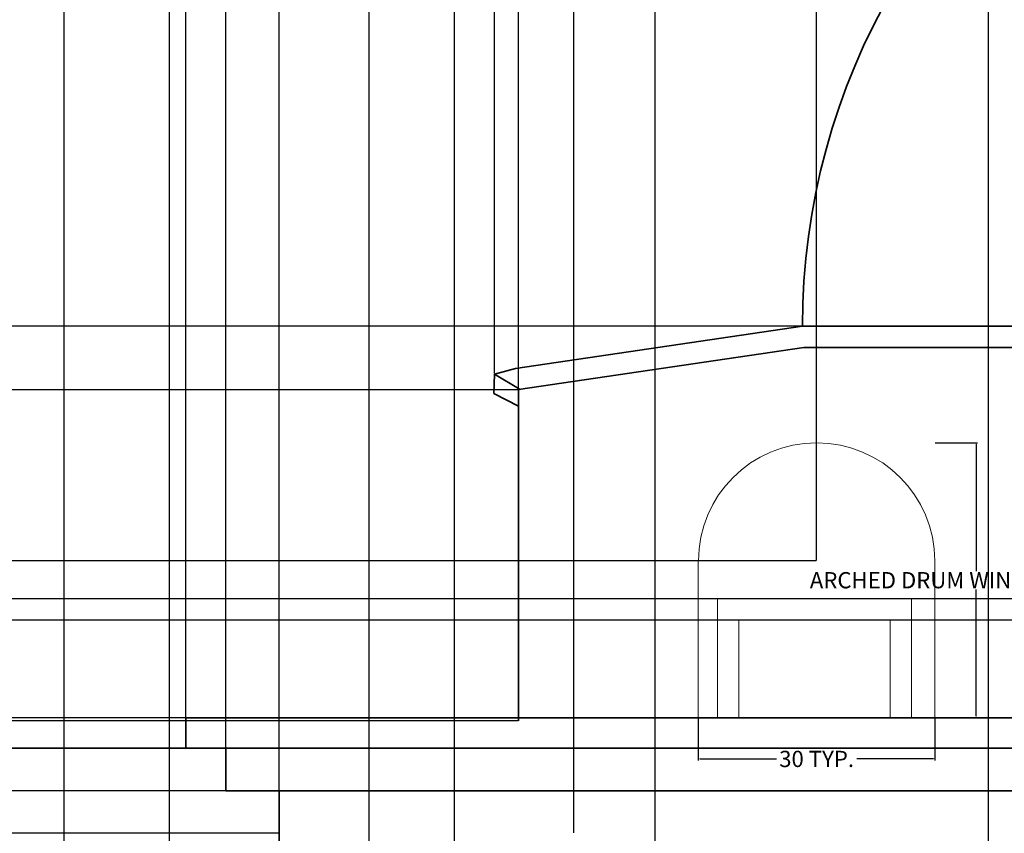
# Model space of a CAD drawing. Units: inches. Extents: x 14 to 859, y 52 to 711.
# Tile 6 of 11: x 244 to 368, y 504 to 608. Entities that reach past the tile are written whole.
import ezdxf

# ---------------------------------------------------------------- set-up
doc = ezdxf.new("R2010")
doc.units = ezdxf.units.IN
doc.header["$MEASUREMENT"] = 0
for name, color, linetype, lineweight in [('A-ANNO-DIMS', 2, 'Continuous', 18), ('A-ELEV', 7, 'Continuous', 35), ('A-GLAZ', 4, 'Continuous', 18), ('A-ROOF', 7, 'Continuous', 35)]:
    doc.layers.add(name, color=color, linetype=linetype, lineweight=lineweight)
doc.styles.get("Standard").update_dxf_attribs({"font": 'arial.ttf'})
doc.dimstyles.get("Standard").update_dxf_attribs({"dimtxt": 2.0625, "dimasz": 0.18, "dimexe": 0.18, "dimexo": 0.0625, "dimgap": 0.09, "dimtad": 0, "dimtih": 1, "dimtoh": 1, "dimdec": 4, "dimzin": 0, "dimdsep": 46, "dimlunit": 4, "dimtxsty": 'Standard', "dimcen": 0.09, "dimadec": 0, "dimazin": 0, "dimtfac": 1, "dimtdec": 4, "dimtofl": 0, "dimtmove": 0, "dimatfit": 3, "dimfxl": 1, "dimtolj": 1, "dimtzin": 0, "dimarcsym": 0})

# ---------------------------------------------------------------- blocks, each defined once
blk = doc.blocks.new('WIN-DRUM-ARCHED')
for p, q in [((329.67, 519.05), (329.67, 538.94)), ((359.68, 519.05), (359.68, 538.94))]:
    blk.add_line(p, q)
for points in [[(332.09, 519.05), (332.09, 534.15), (356.71, 534.15), (356.71, 519.05)], [(334.8, 519.05), (334.8, 531.45), (354.01, 531.45), (354.01, 519.05)]]:
    blk.add_lwpolyline(points)
blk.add_arc((344.68, 538.94), 15, 0, 180)
blk = doc.blocks.new('*D11')
at = {"layer": 'A-ANNO-DIMS', "color": 0, "lineweight": -2, "transparency": 16777216}
for p, q in [((359.74, 553.94), (365.09, 553.94)), ((364.91, 553.76), (364.91, 537.66)), ((364.91, 519.23), (364.91, 535.34)), ((359.74, 519.05), (365.09, 519.05))]:
    blk.add_line(p, q, dxfattribs=at)
at = {"layer": 'A-ANNO-DIMS', "color": 0, "transparency": 16777216}
for points in [[(364.88, 553.76), (364.94, 553.76), (364.91, 553.94)], [(364.88, 519.23), (364.94, 519.23), (364.91, 519.05)]]:
    blk.add_solid(points, dxfattribs=at)
at = {"layer": 'Defpoints', "color": 0, "transparency": 16777216}
for p in [(359.68, 553.94), (364.91, 553.94), (359.68, 519.05)]:
    blk.add_point(p, dxfattribs=at)
at = {"layer": 'A-ANNO-DIMS', "color": 0, "transparency": 16777216, "insert": (364.91, 536.5), "char_height": 2.0625, "attachment_point": 5}
blk.add_mtext('\\A1;ARCHED DRUM WINDOW 35 TYP.', dxfattribs=at)
blk = doc.blocks.new('*D12')
at = {"layer": 'A-ANNO-DIMS', "color": 0, "lineweight": -2, "transparency": 16777216}
for p, q in [((329.67, 518.99), (329.67, 513.64)), ((359.68, 518.99), (359.68, 513.64)), ((329.85, 513.82), (339.57, 513.82)), ((359.5, 513.82), (349.79, 513.82))]:
    blk.add_line(p, q, dxfattribs=at)
at = {"layer": 'A-ANNO-DIMS', "color": 0, "transparency": 16777216}
for points in [[(329.85, 513.85), (329.85, 513.79), (329.67, 513.82)], [(359.5, 513.85), (359.5, 513.79), (359.68, 513.82)]]:
    blk.add_solid(points, dxfattribs=at)
at = {"layer": 'Defpoints', "color": 0, "transparency": 16777216}
for p in [(329.67, 519.05), (359.68, 519.05), (359.68, 513.82)]:
    blk.add_point(p, dxfattribs=at)
at = {"layer": 'A-ANNO-DIMS', "color": 0, "transparency": 16777216, "insert": (344.68, 513.82), "char_height": 2.0625, "attachment_point": 5}
blk.add_mtext('\\A1;30 TYP.', dxfattribs=at)
blk = doc.blocks.new('*D13')
at = {"layer": 'A-ANNO-DIMS', "color": 0, "lineweight": -2, "transparency": 16777216}
for p, q in [((60.78, 339.73), (60.78, 709.71)), ((811.55, 339.73), (811.55, 709.71)), ((60.96, 709.53), (432.6, 709.53)), ((811.37, 709.53), (439.73, 709.53))]:
    blk.add_line(p, q, dxfattribs=at)
at = {"layer": 'A-ANNO-DIMS', "color": 0, "transparency": 16777216}
for points in [[(60.96, 709.56), (60.96, 709.5), (60.78, 709.53)], [(811.37, 709.56), (811.37, 709.5), (811.55, 709.53)]]:
    blk.add_solid(points, dxfattribs=at)
at = {"layer": 'Defpoints', "color": 0, "transparency": 16777216}
for p in [(811.55, 709.53), (60.78, 339.66), (811.55, 339.66)]:
    blk.add_point(p, dxfattribs=at)
at = {"layer": 'A-ANNO-DIMS', "color": 0, "transparency": 16777216, "insert": (436.17, 709.53), "char_height": 2.062, "attachment_point": 5}
blk.add_mtext('\\A1;750.8', dxfattribs=at)
blk = doc.blocks.new('*D16')
at = {"layer": 'A-ANNO-DIMS', "color": 0, "lineweight": -2, "transparency": 16777216}
for p, q in [((429.96, 670.76), (17.7, 670.76)), ((17.88, 670.58), (17.88, 384.41)), ((17.88, 95.97), (17.88, 382.14)), ((60.72, 95.79), (17.7, 95.79))]:
    blk.add_line(p, q, dxfattribs=at)
at = {"layer": 'A-ANNO-DIMS', "color": 0, "transparency": 16777216}
for points in [[(17.85, 670.58), (17.91, 670.58), (17.88, 670.76)], [(17.85, 95.97), (17.91, 95.97), (17.88, 95.79)]]:
    blk.add_solid(points, dxfattribs=at)
at = {"layer": 'Defpoints', "color": 0, "transparency": 16777216}
for p in [(17.88, 670.76), (430.02, 670.76), (60.78, 95.79)]:
    blk.add_point(p, dxfattribs=at)
at = {"layer": 'A-ANNO-DIMS', "color": 0, "transparency": 16777216, "insert": (17.88, 383.28), "char_height": 2.062, "attachment_point": 5}
blk.add_mtext('\\A1;575', dxfattribs=at)
blk = doc.blocks.new('*D21')
at = {"layer": 'A-ANNO-DIMS', "color": 0, "lineweight": -2, "transparency": 16777216}
for p, q in [((287.89, 352.49), (287.89, 709.71)), ((298.73, 341.73), (298.73, 709.71)), ((288.07, 709.53), (289.04, 709.53)), ((298.55, 709.53), (297.59, 709.53))]:
    blk.add_line(p, q, dxfattribs=at)
at = {"layer": 'A-ANNO-DIMS', "color": 0, "transparency": 16777216}
for points in [[(288.07, 709.56), (288.07, 709.5), (287.89, 709.53)], [(298.55, 709.56), (298.55, 709.5), (298.73, 709.53)]]:
    blk.add_solid(points, dxfattribs=at)
at = {"layer": 'Defpoints', "color": 0, "transparency": 16777216}
for p in [(298.73, 709.53), (287.89, 352.43), (298.73, 341.67)]:
    blk.add_point(p, dxfattribs=at)
at = {"layer": 'A-ANNO-DIMS', "color": 0, "transparency": 16777216, "insert": (293.31, 709.53), "char_height": 2.062, "attachment_point": 5}
blk.add_mtext('\\A1;10.837', dxfattribs=at)
blk = doc.blocks.new('*D22')
at = {"layer": 'A-ANNO-DIMS', "color": 0, "lineweight": -2, "transparency": 16777216}
for p, q in [((298.73, 341.73), (298.73, 709.71)), ((576.51, 341.73), (576.51, 709.71)), ((298.91, 709.53), (434.03, 709.53)), ((576.33, 709.53), (441.21, 709.53))]:
    blk.add_line(p, q, dxfattribs=at)
at = {"layer": 'A-ANNO-DIMS', "color": 0, "transparency": 16777216}
for points in [[(298.91, 709.56), (298.91, 709.5), (298.73, 709.53)], [(576.33, 709.56), (576.33, 709.5), (576.51, 709.53)]]:
    blk.add_solid(points, dxfattribs=at)
at = {"layer": 'Defpoints', "color": 0, "transparency": 16777216}
for p in [(576.51, 709.53), (298.73, 341.67), (576.51, 341.67)]:
    blk.add_point(p, dxfattribs=at)
at = {"layer": 'A-ANNO-DIMS', "color": 0, "transparency": 16777216, "insert": (437.62, 709.53), "char_height": 2.062, "attachment_point": 5}
blk.add_mtext('\\A1;277.8', dxfattribs=at)
blk = doc.blocks.new('*D66')
at = {"layer": 'A-ANNO-DIMS', "color": 0, "lineweight": -2, "transparency": 16777216}
for p, q in [((223.53, 404.43), (223.53, 709.71)), ((249.19, 404.43), (249.19, 709.71)), ((223.71, 709.53), (232.77, 709.53)), ((249.01, 709.53), (239.95, 709.53))]:
    blk.add_line(p, q, dxfattribs=at)
at = {"layer": 'A-ANNO-DIMS', "color": 0, "transparency": 16777216}
for points in [[(223.71, 709.56), (223.71, 709.5), (223.53, 709.53)], [(249.01, 709.56), (249.01, 709.5), (249.19, 709.53)]]:
    blk.add_solid(points, dxfattribs=at)
at = {"layer": 'Defpoints', "color": 0, "transparency": 16777216}
for p in [(249.19, 709.53), (223.53, 404.37), (249.19, 404.37)]:
    blk.add_point(p, dxfattribs=at)
at = {"layer": 'A-ANNO-DIMS', "color": 0, "transparency": 16777216, "insert": (236.36, 709.53), "char_height": 2.062, "attachment_point": 5}
blk.add_mtext('\\A1;25.67', dxfattribs=at)
blk = doc.blocks.new('*D67')
at = {"layer": 'A-ANNO-DIMS', "color": 0, "lineweight": -2, "transparency": 16777216}
for p, q in [((249.19, 404.43), (249.19, 709.71)), ((262.58, 404.43), (262.58, 709.71)), ((249.37, 709.53), (252.41, 709.53)), ((262.4, 709.53), (259.36, 709.53))]:
    blk.add_line(p, q, dxfattribs=at)
at = {"layer": 'A-ANNO-DIMS', "color": 0, "transparency": 16777216}
for points in [[(249.37, 709.56), (249.37, 709.5), (249.19, 709.53)], [(262.4, 709.56), (262.4, 709.5), (262.58, 709.53)]]:
    blk.add_solid(points, dxfattribs=at)
at = {"layer": 'Defpoints', "color": 0, "transparency": 16777216}
for p in [(262.58, 709.53), (249.19, 404.37), (262.58, 404.37)]:
    blk.add_point(p, dxfattribs=at)
at = {"layer": 'A-ANNO-DIMS', "color": 0, "transparency": 16777216, "insert": (255.89, 709.53), "char_height": 2.062, "attachment_point": 5}
blk.add_mtext('\\A1;13.39', dxfattribs=at)
blk = doc.blocks.new('*D87')
at = {"layer": 'A-ANNO-DIMS', "color": 0, "lineweight": -2, "transparency": 16777216}
for p, q in [((276.44, 504.38), (17.7, 504.38)), ((17.88, 504.2), (17.88, 476.81)), ((17.88, 447.13), (17.88, 474.52)), ((366.44, 446.95), (17.7, 446.95))]:
    blk.add_line(p, q, dxfattribs=at)
at = {"layer": 'A-ANNO-DIMS', "color": 0, "transparency": 16777216}
for points in [[(17.85, 504.2), (17.91, 504.2), (17.88, 504.38)], [(17.85, 447.13), (17.91, 447.13), (17.88, 446.95)]]:
    blk.add_solid(points, dxfattribs=at)
at = {"layer": 'Defpoints', "color": 0, "transparency": 16777216}
for p in [(17.88, 504.38), (276.5, 504.38), (366.51, 446.95)]:
    blk.add_point(p, dxfattribs=at)
at = {"layer": 'A-ANNO-DIMS', "color": 0, "transparency": 16777216, "insert": (17.88, 475.67), "char_height": 2.062, "attachment_point": 5}
blk.add_mtext('\\A1;57.43', dxfattribs=at)
blk = doc.blocks.new('*D88')
at = {"layer": 'A-ANNO-DIMS', "color": 0, "lineweight": -2, "transparency": 16777216}
for p, q in [((276.44, 509.79), (17.7, 509.79)), ((17.88, 509.61), (17.88, 508.23)), ((17.88, 504.56), (17.88, 505.94)), ((276.44, 504.38), (17.7, 504.38))]:
    blk.add_line(p, q, dxfattribs=at)
at = {"layer": 'A-ANNO-DIMS', "color": 0, "transparency": 16777216}
for points in [[(17.85, 509.61), (17.91, 509.61), (17.88, 509.79)], [(17.85, 504.56), (17.91, 504.56), (17.88, 504.38)]]:
    blk.add_solid(points, dxfattribs=at)
at = {"layer": 'Defpoints', "color": 0, "transparency": 16777216}
for p in [(17.88, 509.79), (276.5, 509.79), (276.5, 504.38)]:
    blk.add_point(p, dxfattribs=at)
at = {"layer": 'A-ANNO-DIMS', "color": 0, "transparency": 16777216, "insert": (17.88, 507.09), "char_height": 2.062, "attachment_point": 5}
blk.add_mtext('\\A1;5.409', dxfattribs=at)
blk = doc.blocks.new('*D89')
at = {"layer": 'A-ANNO-DIMS', "color": 0, "lineweight": -2, "transparency": 16777216}
for p, q in [((269.65, 515.2), (17.7, 515.2)), ((17.88, 515.02), (17.88, 513.64)), ((17.88, 509.97), (17.88, 511.35)), ((269.65, 509.79), (17.7, 509.79))]:
    blk.add_line(p, q, dxfattribs=at)
at = {"layer": 'A-ANNO-DIMS', "color": 0, "transparency": 16777216}
for points in [[(17.85, 515.02), (17.91, 515.02), (17.88, 515.2)], [(17.85, 509.97), (17.91, 509.97), (17.88, 509.79)]]:
    blk.add_solid(points, dxfattribs=at)
at = {"layer": 'Defpoints', "color": 0, "transparency": 16777216}
for p in [(17.88, 515.2), (269.71, 515.2), (269.71, 509.79)]:
    blk.add_point(p, dxfattribs=at)
at = {"layer": 'A-ANNO-DIMS', "color": 0, "transparency": 16777216, "insert": (17.88, 512.49), "char_height": 2.062, "attachment_point": 5}
blk.add_mtext('\\A1;5.409', dxfattribs=at)
blk = doc.blocks.new('*D90')
at = {"layer": 'A-ANNO-DIMS', "color": 0, "lineweight": -2, "transparency": 16777216}
for p, q in [((264.56, 519.05), (17.7, 519.05)), ((17.88, 518.87), (17.88, 518.24)), ((264.56, 515.14), (17.7, 515.14)), ((17.88, 515.32), (17.88, 515.95))]:
    blk.add_line(p, q, dxfattribs=at)
at = {"layer": 'A-ANNO-DIMS', "color": 0, "transparency": 16777216}
for points in [[(17.85, 518.87), (17.91, 518.87), (17.88, 519.05)], [(17.85, 515.32), (17.91, 515.32), (17.88, 515.14)]]:
    blk.add_solid(points, dxfattribs=at)
at = {"layer": 'Defpoints', "color": 0, "transparency": 16777216}
for p in [(17.88, 519.05), (264.63, 519.05), (264.63, 515.14)]:
    blk.add_point(p, dxfattribs=at)
at = {"layer": 'A-ANNO-DIMS', "color": 0, "transparency": 16777216, "insert": (17.88, 517.1), "char_height": 2.062, "attachment_point": 5}
blk.add_mtext('\\A1;3.91', dxfattribs=at)
blk = doc.blocks.new('*D91')
at = {"layer": 'A-ANNO-DIMS', "color": 0, "lineweight": -2, "transparency": 16777216}
for p, q in [((306.8, 560.68), (17.7, 560.68)), ((17.88, 560.5), (17.88, 541.01)), ((17.88, 519.23), (17.88, 538.72)), ((264.56, 519.05), (17.7, 519.05))]:
    blk.add_line(p, q, dxfattribs=at)
at = {"layer": 'A-ANNO-DIMS', "color": 0, "transparency": 16777216}
for points in [[(17.85, 560.5), (17.91, 560.5), (17.88, 560.68)], [(17.85, 519.23), (17.91, 519.23), (17.88, 519.05)]]:
    blk.add_solid(points, dxfattribs=at)
at = {"layer": 'Defpoints', "color": 0, "transparency": 16777216}
for p in [(17.88, 560.68), (306.86, 560.68), (264.63, 519.05)]:
    blk.add_point(p, dxfattribs=at)
at = {"layer": 'A-ANNO-DIMS', "color": 0, "transparency": 16777216, "insert": (17.88, 539.87), "char_height": 2.062, "attachment_point": 5}
blk.add_mtext('\\A1;41.63', dxfattribs=at)
blk = doc.blocks.new('*D92')
at = {"layer": 'A-ANNO-DIMS', "color": 0, "lineweight": -2, "transparency": 16777216}
for p, q in [((342.81, 568.74), (17.7, 568.74)), ((17.88, 568.56), (17.88, 565.85)), ((17.88, 560.86), (17.88, 563.57)), ((306.8, 560.68), (17.7, 560.68))]:
    blk.add_line(p, q, dxfattribs=at)
at = {"layer": 'A-ANNO-DIMS', "color": 0, "transparency": 16777216}
for points in [[(17.85, 568.56), (17.91, 568.56), (17.88, 568.74)], [(17.85, 560.86), (17.91, 560.86), (17.88, 560.68)]]:
    blk.add_solid(points, dxfattribs=at)
at = {"layer": 'Defpoints', "color": 0, "transparency": 16777216}
for p in [(17.88, 568.74), (342.87, 568.74), (306.86, 560.68)]:
    blk.add_point(p, dxfattribs=at)
at = {"layer": 'A-ANNO-DIMS', "color": 0, "transparency": 16777216, "insert": (17.88, 564.71), "char_height": 2.062, "attachment_point": 5}
blk.add_mtext('\\A1;8.055', dxfattribs=at)
blk = doc.blocks.new('*D93')
at = {"layer": 'A-ANNO-DIMS', "color": 0, "lineweight": -2, "transparency": 16777216}
for p, q in [((429.22, 654.01), (17.7, 654.01)), ((17.88, 653.83), (17.88, 612.51)), ((17.88, 568.92), (17.88, 610.23)), ((342.81, 568.74), (17.7, 568.74))]:
    blk.add_line(p, q, dxfattribs=at)
at = {"layer": 'A-ANNO-DIMS', "color": 0, "transparency": 16777216}
for points in [[(17.85, 653.83), (17.91, 653.83), (17.88, 654.01)], [(17.85, 568.92), (17.91, 568.92), (17.88, 568.74)]]:
    blk.add_solid(points, dxfattribs=at)
at = {"layer": 'Defpoints', "color": 0, "transparency": 16777216}
for p in [(17.88, 654.01), (429.29, 654.01), (342.87, 568.74)]:
    blk.add_point(p, dxfattribs=at)
at = {"layer": 'A-ANNO-DIMS', "color": 0, "transparency": 16777216, "insert": (17.88, 611.37), "char_height": 2.062, "attachment_point": 5}
blk.add_mtext('\\A1;85.27', dxfattribs=at)
blk = doc.blocks.new('*D95')
at = {"layer": 'A-ANNO-DIMS', "color": 0, "lineweight": -2, "transparency": 16777216}
for p, q in [((276.5, 504.44), (276.5, 709.71)), ((313.86, 504.44), (313.86, 709.71)), ((276.68, 709.53), (290.81, 709.53)), ((313.68, 709.53), (299.55, 709.53))]:
    blk.add_line(p, q, dxfattribs=at)
at = {"layer": 'A-ANNO-DIMS', "color": 0, "transparency": 16777216}
for points in [[(276.68, 709.56), (276.68, 709.5), (276.5, 709.53)], [(313.68, 709.56), (313.68, 709.5), (313.86, 709.53)]]:
    blk.add_solid(points, dxfattribs=at)
at = {"layer": 'Defpoints', "color": 0, "transparency": 16777216}
for p in [(313.86, 709.53), (276.5, 504.38), (313.86, 504.38)]:
    blk.add_point(p, dxfattribs=at)
at = {"layer": 'A-ANNO-DIMS', "color": 0, "transparency": 16777216, "insert": (295.18, 709.53), "char_height": 2.062, "attachment_point": 5}
blk.add_mtext('\\A1;37.356', dxfattribs=at)
blk = doc.blocks.new('*D96')
at = {"layer": 'A-ANNO-DIMS', "color": 0, "lineweight": -2, "transparency": 16777216}
for p, q in [((313.86, 504.44), (313.86, 709.71)), ((366.51, 447.01), (366.51, 709.71)), ((314.04, 709.53), (336.61, 709.53)), ((366.33, 709.53), (343.76, 709.53))]:
    blk.add_line(p, q, dxfattribs=at)
at = {"layer": 'A-ANNO-DIMS', "color": 0, "transparency": 16777216}
for points in [[(314.04, 709.56), (314.04, 709.5), (313.86, 709.53)], [(366.33, 709.56), (366.33, 709.5), (366.51, 709.53)]]:
    blk.add_solid(points, dxfattribs=at)
at = {"layer": 'Defpoints', "color": 0, "transparency": 16777216}
for p in [(366.51, 709.53), (313.86, 504.38), (366.51, 446.95)]:
    blk.add_point(p, dxfattribs=at)
at = {"layer": 'A-ANNO-DIMS', "color": 0, "transparency": 16777216, "insert": (340.18, 709.53), "char_height": 2.062, "attachment_point": 5}
blk.add_mtext('\\A1;52.65', dxfattribs=at)
blk = doc.blocks.new('*D97')
at = {"layer": 'A-ANNO-DIMS', "color": 0, "lineweight": -2, "transparency": 16777216}
for p, q in [((366.51, 447.01), (366.51, 709.71)), ((433.06, 447.01), (433.06, 709.71)), ((366.69, 709.53), (396.2, 709.53)), ((432.88, 709.53), (403.37, 709.53))]:
    blk.add_line(p, q, dxfattribs=at)
at = {"layer": 'A-ANNO-DIMS', "color": 0, "transparency": 16777216}
for points in [[(366.69, 709.56), (366.69, 709.5), (366.51, 709.53)], [(432.88, 709.56), (432.88, 709.5), (433.06, 709.53)]]:
    blk.add_solid(points, dxfattribs=at)
at = {"layer": 'Defpoints', "color": 0, "transparency": 16777216}
for p in [(433.06, 709.53), (366.51, 446.95), (433.06, 446.95)]:
    blk.add_point(p, dxfattribs=at)
at = {"layer": 'A-ANNO-DIMS', "color": 0, "transparency": 16777216, "insert": (399.78, 709.53), "char_height": 2.062, "attachment_point": 5}
blk.add_mtext('\\A1;66.55', dxfattribs=at)
blk = doc.blocks.new('*D104')
at = {"layer": 'A-ANNO-DIMS', "color": 0, "lineweight": -2, "transparency": 16777216}
for p, q in [((264.63, 519.11), (264.63, 709.71)), ((269.71, 515.26), (269.71, 709.71)), ((264.81, 709.53), (269.53, 709.53)), ((269.71, 709.53), (269.89, 709.53))]:
    blk.add_line(p, q, dxfattribs=at)
at = {"layer": 'A-ANNO-DIMS', "color": 0, "transparency": 16777216}
for points in [[(264.81, 709.56), (264.81, 709.5), (264.63, 709.53)], [(269.53, 709.56), (269.53, 709.5), (269.71, 709.53)]]:
    blk.add_solid(points, dxfattribs=at)
at = {"layer": 'Defpoints', "color": 0, "transparency": 16777216}
for p in [(269.71, 709.53), (264.63, 519.05), (269.71, 515.2)]:
    blk.add_point(p, dxfattribs=at)
at = {"layer": 'A-ANNO-DIMS', "color": 0, "transparency": 16777216, "insert": (273.46, 709.53), "char_height": 2.062, "attachment_point": 5}
blk.add_mtext('\\A1;5.084', dxfattribs=at)
blk = doc.blocks.new('*D105')
at = {"layer": 'A-ANNO-DIMS', "color": 0, "lineweight": -2, "transparency": 16777216}
for p, q in [((306.86, 560.74), (306.86, 709.71)), ((549.44, 560.74), (549.44, 709.71)), ((307.04, 709.53), (424.56, 709.53)), ((549.26, 709.53), (431.74, 709.53))]:
    blk.add_line(p, q, dxfattribs=at)
at = {"layer": 'A-ANNO-DIMS', "color": 0, "transparency": 16777216}
for points in [[(307.04, 709.56), (307.04, 709.5), (306.86, 709.53)], [(549.26, 709.56), (549.26, 709.5), (549.44, 709.53)]]:
    blk.add_solid(points, dxfattribs=at)
at = {"layer": 'Defpoints', "color": 0, "transparency": 16777216}
for p in [(549.44, 709.53), (306.86, 560.68), (549.44, 560.68)]:
    blk.add_point(p, dxfattribs=at)
at = {"layer": 'A-ANNO-DIMS', "color": 0, "transparency": 16777216, "insert": (428.15, 709.53), "char_height": 2.062, "attachment_point": 5}
blk.add_mtext('\\A1;242.6', dxfattribs=at)
blk = doc.blocks.new('*D106')
at = {"layer": 'A-ANNO-DIMS', "color": 0, "lineweight": -2, "transparency": 16777216}
for p, q in [((303.82, 562.72), (303.82, 709.71)), ((306.86, 560.74), (306.86, 709.71)), ((304, 709.53), (306.68, 709.53)), ((306.86, 709.53), (307.04, 709.53))]:
    blk.add_line(p, q, dxfattribs=at)
at = {"layer": 'A-ANNO-DIMS', "color": 0, "transparency": 16777216}
for points in [[(304, 709.56), (304, 709.5), (303.82, 709.53)], [(306.68, 709.56), (306.68, 709.5), (306.86, 709.53)]]:
    blk.add_solid(points, dxfattribs=at)
at = {"layer": 'Defpoints', "color": 0, "transparency": 16777216}
for p in [(306.86, 709.53), (303.82, 562.66), (306.86, 560.68)]:
    blk.add_point(p, dxfattribs=at)
at = {"layer": 'A-ANNO-DIMS', "color": 0, "transparency": 16777216, "insert": (309.8, 709.53), "char_height": 2.062, "attachment_point": 5}
blk.add_mtext('\\A1;3.04', dxfattribs=at)
blk = doc.blocks.new('*D108')
at = {"layer": 'A-ANNO-DIMS', "color": 0, "lineweight": -2, "transparency": 16777216}
for p, q in [((264.63, 519.11), (264.63, 709.71)), ((306.86, 560.74), (306.86, 709.71)), ((264.81, 709.53), (282.13, 709.53)), ((306.68, 709.53), (289.36, 709.53))]:
    blk.add_line(p, q, dxfattribs=at)
at = {"layer": 'A-ANNO-DIMS', "color": 0, "transparency": 16777216}
for points in [[(264.81, 709.56), (264.81, 709.5), (264.63, 709.53)], [(306.68, 709.56), (306.68, 709.5), (306.86, 709.53)]]:
    blk.add_solid(points, dxfattribs=at)
at = {"layer": 'Defpoints', "color": 0, "transparency": 16777216}
for p in [(306.86, 709.53), (306.86, 560.68), (264.63, 519.05)]:
    blk.add_point(p, dxfattribs=at)
at = {"layer": 'A-ANNO-DIMS', "color": 0, "transparency": 16777216, "insert": (285.74, 709.53), "char_height": 2.062, "attachment_point": 5}
blk.add_mtext('\\A1;42.23', dxfattribs=at)
blk = doc.blocks.new('*D109')
at = {"layer": 'A-ANNO-DIMS', "color": 0, "lineweight": -2, "transparency": 16777216}
for p, q in [((269.71, 515.26), (269.71, 709.71)), ((276.5, 509.85), (276.5, 709.71)), ((269.89, 709.53), (276.32, 709.53)), ((276.5, 709.53), (276.68, 709.53))]:
    blk.add_line(p, q, dxfattribs=at)
at = {"layer": 'A-ANNO-DIMS', "color": 0, "transparency": 16777216}
for points in [[(269.89, 709.56), (269.89, 709.5), (269.71, 709.53)], [(276.32, 709.56), (276.32, 709.5), (276.5, 709.53)]]:
    blk.add_solid(points, dxfattribs=at)
at = {"layer": 'Defpoints', "color": 0, "transparency": 16777216}
for p in [(276.5, 709.53), (269.71, 515.2), (276.5, 509.79)]:
    blk.add_point(p, dxfattribs=at)
at = {"layer": 'A-ANNO-DIMS', "color": 0, "transparency": 16777216, "insert": (280.26, 709.53), "char_height": 2.062, "attachment_point": 5}
blk.add_mtext('\\A1;6.793', dxfattribs=at)
blk = doc.blocks.new('*D110')
at = {"layer": 'A-ANNO-DIMS', "color": 0, "lineweight": -2, "transparency": 16777216}
for p, q in [((306.86, 518.73), (306.86, 709.71)), ((344.68, 539), (344.68, 709.71)), ((307.04, 709.53), (322.21, 709.53)), ((344.5, 709.53), (329.33, 709.53))]:
    blk.add_line(p, q, dxfattribs=at)
at = {"layer": 'A-ANNO-DIMS', "color": 0, "transparency": 16777216}
for points in [[(307.04, 709.56), (307.04, 709.5), (306.86, 709.53)], [(344.5, 709.56), (344.5, 709.5), (344.68, 709.53)]]:
    blk.add_solid(points, dxfattribs=at)
at = {"layer": 'Defpoints', "color": 0, "transparency": 16777216}
for p in [(344.68, 709.53), (344.68, 538.94), (306.86, 518.67)]:
    blk.add_point(p, dxfattribs=at)
at = {"layer": 'A-ANNO-DIMS', "color": 0, "transparency": 16777216, "insert": (325.77, 709.53), "char_height": 2.062, "attachment_point": 5}
blk.add_mtext('\\A1;37.82', dxfattribs=at)
blk = doc.blocks.new('*D111')
at = {"layer": 'A-ANNO-DIMS', "color": 0, "lineweight": -2, "transparency": 16777216}
for p, q in [((344.68, 539), (344.68, 709.71)), ((424.02, 539), (424.02, 709.71)), ((344.86, 709.53), (380.79, 709.53)), ((423.84, 709.53), (387.91, 709.53))]:
    blk.add_line(p, q, dxfattribs=at)
at = {"layer": 'A-ANNO-DIMS', "color": 0, "transparency": 16777216}
for points in [[(344.86, 709.56), (344.86, 709.5), (344.68, 709.53)], [(423.84, 709.56), (423.84, 709.5), (424.02, 709.53)]]:
    blk.add_solid(points, dxfattribs=at)
at = {"layer": 'Defpoints', "color": 0, "transparency": 16777216}
for p in [(424.02, 709.53), (344.68, 538.94), (424.02, 538.94)]:
    blk.add_point(p, dxfattribs=at)
at = {"layer": 'A-ANNO-DIMS', "color": 0, "transparency": 16777216, "insert": (384.35, 709.53), "char_height": 2.062, "attachment_point": 5}
blk.add_mtext('\\A1;79.34', dxfattribs=at)
blk = doc.blocks.new('*D113')
at = {"layer": 'A-ANNO-DIMS', "color": 0, "lineweight": -2, "transparency": 16777216}
for p, q in [((344.62, 538.94), (17.7, 538.94)), ((17.88, 538.76), (17.88, 529.95)), ((17.88, 518.85), (17.88, 527.66)), ((306.8, 518.67), (17.7, 518.67))]:
    blk.add_line(p, q, dxfattribs=at)
at = {"layer": 'A-ANNO-DIMS', "color": 0, "transparency": 16777216}
for points in [[(17.85, 538.76), (17.91, 538.76), (17.88, 538.94)], [(17.85, 518.85), (17.91, 518.85), (17.88, 518.67)]]:
    blk.add_solid(points, dxfattribs=at)
at = {"layer": 'Defpoints', "color": 0, "transparency": 16777216}
for p in [(17.88, 538.94), (344.68, 538.94), (306.86, 518.67)]:
    blk.add_point(p, dxfattribs=at)
at = {"layer": 'A-ANNO-DIMS', "color": 0, "transparency": 16777216, "insert": (17.88, 528.81), "char_height": 2.062, "attachment_point": 5}
blk.add_mtext('\\A1;20.273', dxfattribs=at)
blk = doc.blocks.new('*D116')
at = {"layer": 'A-ANNO-DIMS', "color": 0, "lineweight": -2, "transparency": 16777216}
for p, q in [((435.99, 534.15), (17.7, 534.15)), ((17.88, 533.97), (17.88, 527.74)), ((17.88, 519.23), (17.88, 525.46)), ((435.99, 519.05), (17.7, 519.05))]:
    blk.add_line(p, q, dxfattribs=at)
at = {"layer": 'A-ANNO-DIMS', "color": 0, "transparency": 16777216}
for points in [[(17.85, 533.97), (17.91, 533.97), (17.88, 534.15)], [(17.85, 519.23), (17.91, 519.23), (17.88, 519.05)]]:
    blk.add_solid(points, dxfattribs=at)
at = {"layer": 'Defpoints', "color": 0, "transparency": 16777216}
for p in [(17.88, 534.15), (436.05, 534.15), (436.05, 519.05)]:
    blk.add_point(p, dxfattribs=at)
at = {"layer": 'A-ANNO-DIMS', "color": 0, "transparency": 16777216, "insert": (17.88, 526.6), "char_height": 2.062, "attachment_point": 5}
blk.add_mtext('\\A1;15.1', dxfattribs=at)
blk = doc.blocks.new('*D117')
at = {"layer": 'A-ANNO-DIMS', "color": 0, "lineweight": -2, "transparency": 16777216}
for p, q in [((433.29, 531.45), (17.7, 531.45)), ((17.88, 531.27), (17.88, 526.39)), ((17.88, 519.23), (17.88, 524.11)), ((433.29, 519.05), (17.7, 519.05))]:
    blk.add_line(p, q, dxfattribs=at)
at = {"layer": 'A-ANNO-DIMS', "color": 0, "transparency": 16777216}
for points in [[(17.85, 531.27), (17.91, 531.27), (17.88, 531.45)], [(17.85, 519.23), (17.91, 519.23), (17.88, 519.05)]]:
    blk.add_solid(points, dxfattribs=at)
at = {"layer": 'Defpoints', "color": 0, "transparency": 16777216}
for p in [(17.88, 531.45), (433.35, 531.45), (433.35, 519.05)]:
    blk.add_point(p, dxfattribs=at)
at = {"layer": 'A-ANNO-DIMS', "color": 0, "transparency": 16777216, "insert": (17.88, 525.25), "char_height": 2.062, "attachment_point": 5}
blk.add_mtext('\\A1;12.395', dxfattribs=at)
blk = doc.blocks.new('*D118')
at = {"layer": 'A-ANNO-DIMS', "color": 0, "lineweight": -2, "transparency": 16777216}
for p, q in [((306.86, 560.74), (306.86, 709.71)), ((428.15, 568.8), (428.15, 709.71)), ((307.04, 709.53), (364.03, 709.53)), ((427.97, 709.53), (370.98, 709.53))]:
    blk.add_line(p, q, dxfattribs=at)
at = {"layer": 'A-ANNO-DIMS', "color": 0, "transparency": 16777216}
for points in [[(307.04, 709.56), (307.04, 709.5), (306.86, 709.53)], [(427.97, 709.56), (427.97, 709.5), (428.15, 709.53)]]:
    blk.add_solid(points, dxfattribs=at)
at = {"layer": 'Defpoints', "color": 0, "transparency": 16777216}
for p in [(428.15, 709.53), (428.15, 568.74), (306.86, 560.68)]:
    blk.add_point(p, dxfattribs=at)
at = {"layer": 'A-ANNO-DIMS', "color": 0, "transparency": 16777216, "insert": (367.51, 709.53), "char_height": 2.062, "attachment_point": 5}
blk.add_mtext('\\A1;121.3', dxfattribs=at)
blk = doc.blocks.new('*D119')
at = {"layer": 'A-ANNO-DIMS', "color": 0, "lineweight": -2, "transparency": 16777216}
for p, q in [((287.89, 404.43), (287.89, 709.71)), ((324.18, 404.43), (324.18, 709.71)), ((288.07, 709.53), (301.66, 709.53)), ((324, 709.53), (310.41, 709.53))]:
    blk.add_line(p, q, dxfattribs=at)
at = {"layer": 'A-ANNO-DIMS', "color": 0, "transparency": 16777216}
for points in [[(288.07, 709.56), (288.07, 709.5), (287.89, 709.53)], [(324, 709.56), (324, 709.5), (324.18, 709.53)]]:
    blk.add_solid(points, dxfattribs=at)
at = {"layer": 'Defpoints', "color": 0, "transparency": 16777216}
for p in [(324.18, 709.53), (287.89, 404.37), (324.18, 404.37)]:
    blk.add_point(p, dxfattribs=at)
at = {"layer": 'A-ANNO-DIMS', "color": 0, "transparency": 16777216, "insert": (306.04, 709.53), "char_height": 2.062, "attachment_point": 5}
blk.add_mtext('\\A1;36.285', dxfattribs=at)
blk = doc.blocks.new('*D120')
at = {"layer": 'A-ANNO-DIMS', "color": 0, "lineweight": -2, "transparency": 16777216}
for p, q in [((324.18, 404.43), (324.18, 709.71)), ((390.73, 404.43), (390.73, 709.71)), ((324.36, 709.53), (353.87, 709.53)), ((390.55, 709.53), (361.04, 709.53))]:
    blk.add_line(p, q, dxfattribs=at)
at = {"layer": 'A-ANNO-DIMS', "color": 0, "transparency": 16777216}
for points in [[(324.36, 709.56), (324.36, 709.5), (324.18, 709.53)], [(390.55, 709.56), (390.55, 709.5), (390.73, 709.53)]]:
    blk.add_solid(points, dxfattribs=at)
at = {"layer": 'Defpoints', "color": 0, "transparency": 16777216}
for p in [(390.73, 709.53), (324.18, 404.37), (390.73, 404.37)]:
    blk.add_point(p, dxfattribs=at)
at = {"layer": 'A-ANNO-DIMS', "color": 0, "transparency": 16777216, "insert": (357.45, 709.53), "char_height": 2.062, "attachment_point": 5}
blk.add_mtext('\\A1;66.55', dxfattribs=at)

msp = doc.modelspace()

# ---------------------------------------------------------------- linework, layer by layer
at = {"layer": 'A-ELEV'}
for p, q in [((306.4653, 563.3562), (342.8739, 568.7358)), ((342.8739, 568.7358), (434.8803, 568.7358)), ((306.8606, 560.6808), (343.0726, 566.0314)), ((343.0726, 566.0314), (434.8803, 566.0314)), ((303.8209, 562.6585), (303.7161, 560.1811)), ((306.4653, 563.3562), (303.8209, 562.6585)), ((303.8209, 562.6585), (307.0757, 560.7126)), ((303.7161, 560.1811), (306.8606, 558.5789)), ((306.8606, 551.9063), (306.8606, 560.6808)), ((306.8606, 518.6693), (306.8606, 551.9063)), ((264.6274, 515.1437), (264.6274, 519.0512)), ((264.6274, 519.0512), (555.2103, 519.0512)), ((269.7112, 515.1991), (264.6274, 515.1437)), ((276.5038, 515.1991), (269.7112, 515.1991)), ((269.7112, 515.1991), (269.7112, 509.7903)), ((276.5038, 515.1991), (537.6873, 515.1991)), ((269.7112, 509.7903), (269.7112, 509.7903)), ((269.7112, 509.7903), (276.5038, 509.7903)), ((276.5038, 405.9412), (276.5038, 509.7903)), ((276.5038, 509.7903), (537.6873, 509.7903))]:
    msp.add_line(p, q, dxfattribs=at)
at = {"layer": 'A-ROOF'}
msp.add_arc((428.1517, 568.7358), 85.2778, 358.475544, 180, dxfattribs=at)

# ---------------------------------------------------------------- block references
at = {"layer": 'A-GLAZ'}
msp.add_blockref('WIN-DRUM-ARCHED', (0, 0), dxfattribs=at)

# ---------------------------------------------------------------- dimensions: what is measured, and where the dimension line sits
at = {"layer": 'A-ANNO-DIMS'}
for base, p1, p2, override, picture, middle in [((811.5534, 709.5262), (60.7804, 339.6626), (811.5534, 339.6626), {"dimdec": 1, "dimlfac": 1, "dimrnd": 0, "dimzin": 0, "dimdsep": 46, "dimlunit": 2}, '*D13', (436.1669, 709.5262)), ((249.1939, 709.5262), (223.5256, 404.3712), (249.1939, 404.3712), {"dimdec": 2, "dimlfac": 1, "dimrnd": 0, "dimzin": 0, "dimdsep": 46, "dimlunit": 2}, '*D66', (236.3598, 709.5262)), ((262.5837, 709.5262), (249.1939, 404.3712), (262.5837, 404.3712), {"dimdec": 2, "dimlfac": 1, "dimrnd": 0, "dimzin": 0, "dimdsep": 46, "dimlunit": 2}, '*D67', (255.8888, 709.5262)), ((269.7112, 709.5262), (264.6274, 519.0512), (269.7112, 515.1991), {"dimdec": 3, "dimlfac": 1, "dimrnd": 0, "dimzin": 0, "dimdsep": 46, "dimlunit": 2}, '*D104', (273.457, 709.5262)), ((306.8606, 709.5262), (264.6274, 519.0512), (306.8606, 560.6808), {"dimdec": 2, "dimlfac": 1, "dimrnd": 0, "dimzin": 0, "dimdsep": 46, "dimlunit": 2}, '*D108', (285.744, 709.5262)), ((276.5038, 709.5262), (269.7112, 515.1991), (276.5038, 509.7903), {"dimdec": 3, "dimlfac": 1, "dimrnd": 0, "dimzin": 0, "dimdsep": 46, "dimlunit": 2}, '*D109', (280.2593, 709.5262)), ((313.8595, 709.5262), (276.5038, 504.3815), (313.8595, 504.3815), {"dimdec": 3, "dimlfac": 1, "dimrnd": 0, "dimzin": 0, "dimdsep": 46, "dimlunit": 2}, '*D95', (295.1816, 709.5262)), ((298.72949, 709.52622), (287.89298, 352.42914), (298.72949, 341.67161), {"dimdec": 3, "dimlfac": 1, "dimrnd": 0, "dimzin": 0, "dimdsep": 46, "dimlunit": 2}, '*D21', (293.31124, 709.52622)), ((324.1777, 709.5262), (287.893, 404.3712), (324.1777, 404.3712), {"dimdec": 3, "dimlfac": 1, "dimrnd": 0, "dimzin": 0, "dimdsep": 46, "dimlunit": 2}, '*D119', (306.0353, 709.5262)), ((576.5058, 709.5262), (298.7295, 341.6716), (576.5058, 341.6716), {"dimdec": 1, "dimlfac": 1, "dimrnd": 0, "dimzin": 0, "dimdsep": 46, "dimlunit": 2}, '*D22', (437.6176, 709.5262)), ((306.8606, 709.5262), (303.8209, 562.6585), (306.8606, 560.6808), {"dimdec": 2, "dimlfac": 1, "dimrnd": 0, "dimzin": 0, "dimdsep": 46, "dimlunit": 2}, '*D106', (309.8044, 709.5262)), ((549.4429, 709.5262), (306.8606, 560.6808), (549.4429, 560.6808), {"dimdec": 1, "dimlfac": 1, "dimrnd": 0, "dimzin": 0, "dimdsep": 46, "dimlunit": 2}, '*D105', (428.1517, 709.5262)), ((344.6778, 709.5262), (306.8606, 518.6693), (344.6778, 538.9419), {"dimdec": 2, "dimlfac": 1, "dimrnd": 0, "dimzin": 0, "dimdsep": 46, "dimlunit": 2}, '*D110', (325.7692, 709.5262)), ((428.1517, 709.5262), (306.8606, 560.6808), (428.1517, 568.7358), {"dimdec": 1, "dimlfac": 1, "dimrnd": 0, "dimzin": 0, "dimdsep": 46, "dimlunit": 2}, '*D118', (367.5062, 709.5262)), ((366.507, 709.5262), (313.8595, 504.3815), (366.507, 446.9501), {"dimdec": 2, "dimlfac": 1, "dimrnd": 0, "dimzin": 0, "dimdsep": 46, "dimlunit": 2}, '*D96', (340.1833, 709.5262)), ((390.7307, 709.5262), (324.1777, 404.3712), (390.7307, 404.3712), {"dimdec": 2, "dimlfac": 1, "dimrnd": 0, "dimzin": 0, "dimdsep": 46, "dimlunit": 2}, '*D120', (357.4542, 709.5262)), ((424.0193, 709.5262), (344.6778, 538.9419), (424.0193, 538.9419), {"dimdec": 2, "dimlfac": 1, "dimrnd": 0, "dimzin": 0, "dimdsep": 46, "dimlunit": 2}, '*D111', (384.3486, 709.5262)), ((433.06, 709.5262), (366.507, 446.9501), (433.06, 446.9501), {"dimdec": 2, "dimlfac": 1, "dimrnd": 0, "dimzin": 0, "dimdsep": 46, "dimlunit": 2}, '*D97', (399.7835, 709.5262))]:
    dim = msp.add_linear_dim(base=base, p1=p1, p2=p2, dimstyle='Standard', override=override, dxfattribs=at)
    dim.commit()
    dim.dimension.update_dxf_attribs({"geometry": picture, "text_midpoint": middle})
for base, p1, p2, override, picture, middle in [((17.8785, 670.7637), (60.7804, 95.7876), (430.0228, 670.7637), {"dimdec": 0, "dimlfac": 1, "dimrnd": 0, "dimzin": 0, "dimdsep": 46, "dimlunit": 2}, '*D16', (17.8785, 383.2756)), ((17.8785, 654.0061), (342.8739, 568.7358), (429.2862, 654.0061), {"dimdec": 2, "dimlfac": 1, "dimrnd": 0, "dimzin": 0, "dimdsep": 46, "dimlunit": 2}, '*D93', (17.8785, 611.371)), ((17.8785, 568.7358), (306.8606, 560.6808), (342.8739, 568.7358), {"dimdec": 3, "dimlfac": 1, "dimrnd": 0, "dimzin": 0, "dimdsep": 46, "dimlunit": 2}, '*D92', (17.8785, 564.7083)), ((17.8785, 560.6808), (264.6274, 519.0512), (306.8606, 560.6808), {"dimdec": 2, "dimlfac": 1, "dimrnd": 0, "dimzin": 0, "dimdsep": 46, "dimlunit": 2}, '*D91', (17.8785, 539.866)), ((17.8785, 538.9419), (306.8606, 518.6693), (344.6778, 538.9419), {"dimdec": 3, "dimlfac": 1, "dimrnd": 0, "dimzin": 0, "dimdsep": 46, "dimlunit": 2}, '*D113', (17.8785, 528.8056)), ((17.8785, 534.1509), (436.0547, 519.0512), (436.0547, 534.1509), {"dimdec": 1, "dimlfac": 1, "dimrnd": 0, "dimzin": 0, "dimdsep": 46, "dimlunit": 2}, '*D116', (17.8785, 526.601)), ((17.8785, 531.4465), (433.3504, 519.0512), (433.3504, 531.4465), {"dimdec": 3, "dimlfac": 1, "dimrnd": 0, "dimzin": 0, "dimdsep": 46, "dimlunit": 2}, '*D117', (17.8785, 525.2488)), ((17.8785, 519.0512), (264.6274, 515.1437), (264.6274, 519.0512), {"dimdec": 2, "dimlfac": 1, "dimrnd": 0, "dimzin": 0, "dimdsep": 46, "dimlunit": 2}, '*D90', (17.8785, 517.0975)), ((17.8785, 515.1991), (269.7112, 509.7903), (269.7112, 515.1991), {"dimdec": 3, "dimlfac": 1, "dimrnd": 0, "dimzin": 0, "dimdsep": 46, "dimlunit": 2}, '*D89', (17.8785, 512.4947)), ((17.8785, 509.7903), (276.5038, 504.3815), (276.5038, 509.7903), {"dimdec": 3, "dimlfac": 1, "dimrnd": 0, "dimzin": 0, "dimdsep": 46, "dimlunit": 2}, '*D88', (17.8785, 507.0859)), ((17.8785, 504.3815), (366.507, 446.9501), (276.5038, 504.3815), {"dimdec": 2, "dimlfac": 1, "dimrnd": 0, "dimzin": 0, "dimdsep": 46, "dimlunit": 2}, '*D87', (17.8785, 475.6658))]:
    dim = msp.add_linear_dim(base=base, p1=p1, p2=p2, angle=90, dimstyle='Standard', override=override, dxfattribs=at)
    dim.commit()
    dim.dimension.update_dxf_attribs({"geometry": picture, "text_midpoint": middle})
dim = msp.add_linear_dim(base=(364.9147, 553.9447), p1=(359.6807, 519.0512), p2=(359.6807, 553.9447), angle=90, text='ARCHED DRUM WINDOW <> TYP.', dimstyle='Standard', override={"dimdec": 0, "dimlfac": 1, "dimrnd": 0, "dimzin": 0, "dimdsep": 46, "dimlunit": 2}, dxfattribs=at)
dim.commit()
dim.dimension.update_dxf_attribs({"geometry": '*D11', "text_midpoint": (364.9147, 536.498)})
dim = msp.add_linear_dim(base=(359.6807, 513.8171), p1=(329.675, 519.0512), p2=(359.6807, 519.0512), text='<> TYP.', dimstyle='Standard', override={"dimdec": 0, "dimlfac": 1, "dimrnd": 0, "dimzin": 0, "dimdsep": 46, "dimlunit": 2}, dxfattribs=at)
dim.commit()
dim.dimension.update_dxf_attribs({"geometry": '*D12', "text_midpoint": (344.6778, 513.8171)})

doc.saveas('drawing.dxf')
